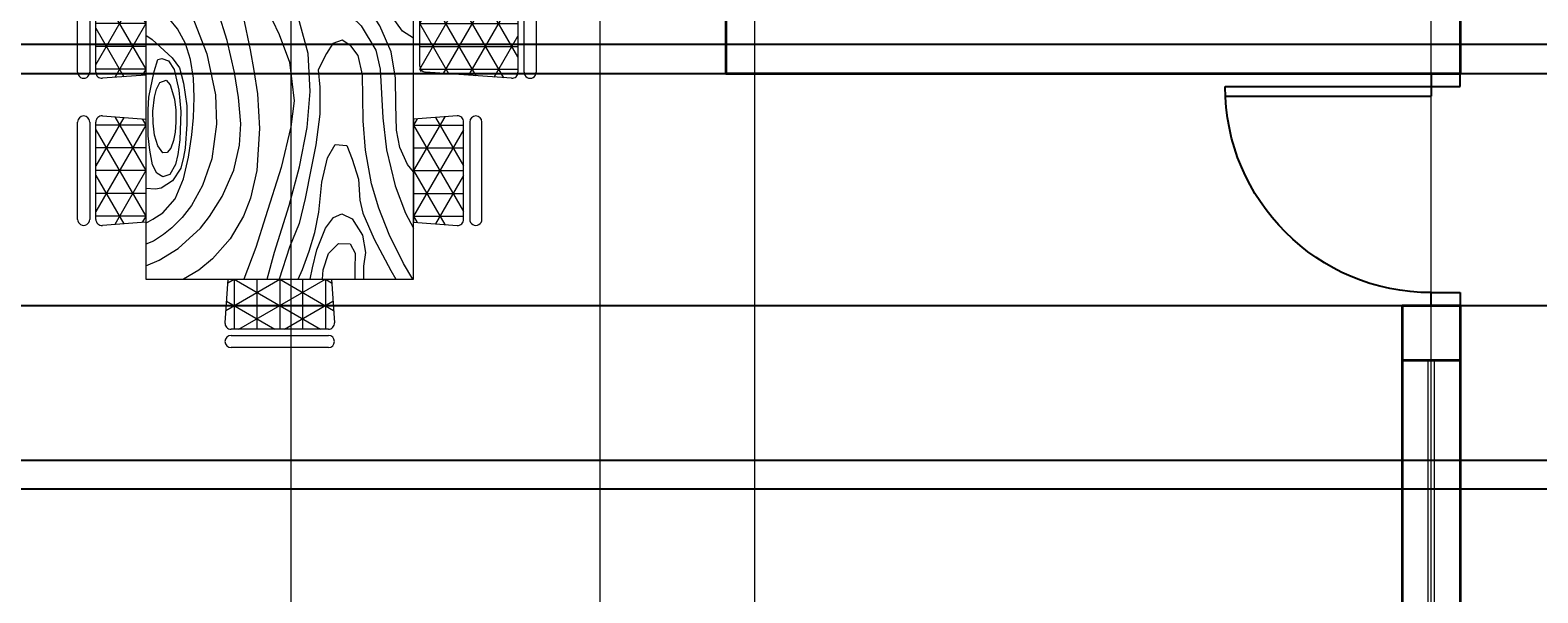
# Model space of a CAD drawing. Units: inches. Extents: x 5716 to 6907, y 12769 to 13594.
# Tile 14 of 17: x 6414 to 6648, y 13105 to 13192. Entities that reach past the tile are written whole.
import ezdxf

# ---------------------------------------------------------------- set-up
doc = ezdxf.new("R2010")
doc.units = ezdxf.units.IN
for name, color, linetype, lineweight in [('A-ANNO-DIMS', 2, 'Continuous', 18), ('A-DOOR', 4, 'Continuous', 25), ('A-FURN', 8, 'Continuous', 18), ('A-GLAZ', 4, 'Continuous', 18), ('A-GRID', 8, 'Continuous', 13), ('A-WALL', 7, 'Continuous', 35)]:
    doc.layers.add(name, color=color, linetype=linetype, lineweight=lineweight)
doc.styles.get("Standard").update_dxf_attribs({"font": 'arial.ttf'})
doc.dimstyles.get("Standard").update_dxf_attribs({"dimtxt": 0.18, "dimasz": 0.18, "dimexe": 0.18, "dimexo": 0.0625, "dimgap": 0.09, "dimtad": 0, "dimtih": 1, "dimtoh": 1, "dimdec": 4, "dimzin": 0, "dimdsep": 46, "dimtxsty": 'Standard', "dimcen": 0.09, "dimadec": 0, "dimazin": 0, "dimtfac": 1, "dimtdec": 4, "dimtofl": 0, "dimtmove": 0, "dimatfit": 3, "dimfxl": 1, "dimtolj": 1, "dimtzin": 0, "dimarcsym": 0})

# ---------------------------------------------------------------- blocks, each defined once
blk = doc.blocks.new('A$C405465A0')
for p, q in [((1.1305, 2.1034), (1.5301, 2.1034)), ((1.5301, 2.0534), (1.1305, 2.0534)), ((1.1304, 1.6481), (1.1055, 2.0017)), ((1.279, 2.0284), (1.1105, 1.9312)), ((1.4665, 2.0284), (1.1178, 1.8271)), ((1.1305, 2.0284), (1.5301, 2.0284)), ((1.1428, 1.625), (1.1428, 2.0284)), ((1.5427, 1.8271), (1.1941, 2.0284)), ((1.2365, 1.625), (1.2365, 2.0284)), ((1.3303, 1.625), (1.3303, 2.0284)), ((1.5501, 1.9312), (1.3816, 2.0284)), ((1.424, 1.625), (1.424, 2.0284)), ((1.5178, 1.625), (1.5178, 2.0284)), ((1.555, 2.0017), (1.5301, 1.6481)), ((1.5354, 1.7231), (1.1078, 1.97)), ((1.5528, 1.97), (1.1252, 1.7231)), ((0.9452, 1.8803), (0.5455, 1.8803)), ((2.1342, 1.8803), (1.7345, 1.8803)), ((0.5268, 1.6904), (0.7259, 1.8053)), ((0.5455, 1.8303), (0.9452, 1.8303)), ((0.9452, 1.8053), (0.5455, 1.8053)), ((0.5578, 1.6), (0.5578, 1.8053)), ((0.5578, 1.6), (0.9134, 1.8053)), ((0.5773, 1.8053), (0.9328, 1.6)), ((0.6516, 1.6), (0.6516, 1.8053)), ((0.7453, 1.6), (0.7453, 1.8053)), ((0.7648, 1.8053), (0.9639, 1.6904)), ((0.8391, 1.6), (0.8391, 1.8053)), ((0.9328, 1.6), (0.9328, 1.8053)), ((1.5178, 1.625), (1.1157, 1.8572)), ((1.5449, 1.8572), (1.1428, 1.625)), ((1.7158, 1.6904), (1.9149, 1.8053)), ((1.7345, 1.8303), (2.1342, 1.8303)), ((2.1342, 1.8053), (1.7345, 1.8053)), ((1.7468, 1.6), (1.7468, 1.8053)), ((1.7468, 1.6), (2.1024, 1.8053)), ((1.7663, 1.8053), (2.1218, 1.6)), ((1.8406, 1.6), (1.8406, 1.8053)), ((1.9343, 1.6), (1.9343, 1.8053)), ((1.9538, 1.8053), (2.1529, 1.6904)), ((2.0281, 1.6), (2.0281, 1.8053)), ((2.1218, 1.6), (2.1218, 1.8053)), ((0.5206, 1.7786), (0.5332, 1.6)), ((0.9575, 1.6), (0.9701, 1.7786)), ((1.3303, 1.625), (1.1237, 1.7443)), ((1.5369, 1.7443), (1.3303, 1.625)), ((1.7096, 1.7786), (1.7222, 1.6)), ((2.1465, 1.6), (2.1591, 1.7786)), ((0.5242, 1.7277), (0.7453, 1.6)), ((0.7453, 1.6), (0.9665, 1.7277)), ((1.7132, 1.7277), (1.9343, 1.6)), ((1.9343, 1.6), (2.1555, 1.7277)), ((0.5321, 1.6149), (0.5578, 1.6)), ((0.9328, 1.6), (0.9586, 1.6149)), ((1.1428, 1.625), (1.1316, 1.6315)), ((1.5052, 1.625), (1.1554, 1.625)), ((1.529, 1.6315), (1.5178, 1.625)), ((1.7211, 1.6149), (1.7468, 1.6)), ((2.1218, 1.6), (2.1476, 1.6149)), ((2.3803, 1.6), (0.2803, 1.6)), ((0.2803, 1.6), (0.2803, 0.5)), ((0.3956, 1.553), (0.3856, 1.5163)), ((0.4356, 1.5842), (0.3956, 1.553)), ((0.5827, 1.5379), (0.4356, 1.5842)), ((0.5332, 1.6), (0.9575, 1.6)), ((0.7152, 1.6), (0.7236, 1.5766)), ((0.7236, 1.5766), (0.7578, 1.4998)), ((0.9055, 1.5469), (0.8836, 1.6)), ((1.0212, 1.6), (1.0194, 1.5656)), ((1.0194, 1.5656), (1.026, 1.5003)), ((1.1178, 1.5243), (1.1269, 1.5706)), ((1.1269, 1.5706), (1.1432, 1.6)), ((1.1887, 1.5196), (1.1922, 1.5507)), ((1.1922, 1.5507), (1.214, 1.6)), ((1.3616, 1.5541), (1.3027, 1.5125)), ((1.3907, 1.6), (1.3616, 1.5541)), ((1.7222, 1.6), (2.1465, 1.6)), ((1.9093, 1.5754), (1.8386, 1.5427)), ((1.9386, 1.6), (1.9093, 1.5754)), ((1.9962, 1.5248), (2.1086, 1.5664)), ((2.1086, 1.5664), (2.17, 1.6)), ((2.3153, 1.558), (2.1962, 1.4994)), ((2.3803, 1.5967), (2.3153, 1.558)), ((2.3803, 0.5), (2.3803, 1.6)), ((0.3856, 1.5163), (0.4538, 1.4363)), ((0.4482, 1.5094), (0.4582, 1.5336)), ((0.4595, 1.4847), (0.4482, 1.5094)), ((0.4582, 1.5336), (0.5016, 1.5339)), ((0.5016, 1.5339), (0.54, 1.5204)), ((0.54, 1.5204), (0.5786, 1.5)), ((0.5786, 1.5), (0.6151, 1.4744)), ((0.6365, 1.5019), (0.5827, 1.5379)), ((0.7193, 1.4377), (0.6365, 1.5019)), ((0.7578, 1.4998), (0.7752, 1.4525)), ((0.9296, 1.4669), (0.9055, 1.5469)), ((1.026, 1.5003), (1.0343, 1.4559)), ((1.1128, 1.4699), (1.1178, 1.5243)), ((1.2089, 1.4946), (1.1887, 1.5196)), ((1.2618, 1.4976), (1.2089, 1.4946)), ((1.3027, 1.5125), (1.2618, 1.4976)), ((1.446, 1.5079), (1.3392, 1.4609)), ((1.5543, 1.5261), (1.446, 1.5079)), ((1.6627, 1.5271), (1.5543, 1.5261)), ((1.7679, 1.5301), (1.6627, 1.5271)), ((1.717, 1.474), (1.8488, 1.4892)), ((1.8386, 1.5427), (1.7679, 1.5301)), ((1.8488, 1.4892), (1.9962, 1.5248)), ((2.1962, 1.4994), (2.0887, 1.4564)), ((2.215, 1.4381), (2.3447, 1.5068)), ((2.3447, 1.5068), (2.3803, 1.5269)), ((0.3744, 1.3943), (0.2803, 1.458)), ((0.4538, 1.4363), (0.5034, 1.394)), ((0.4876, 1.4521), (0.4595, 1.4847)), ((0.5099, 1.4328), (0.4876, 1.4521)), ((0.5366, 1.4137), (0.5099, 1.4328)), ((0.6151, 1.4744), (0.6557, 1.4351)), ((0.6557, 1.4351), (0.6746, 1.4025)), ((0.7442, 1.4091), (0.7193, 1.4377)), ((0.7752, 1.4525), (0.7871, 1.4053)), ((0.9436, 1.385), (0.9296, 1.4669)), ((1.0343, 1.4559), (1.0488, 1.3883)), ((1.1133, 1.4295), (1.1128, 1.4699)), ((1.1222, 1.3821), (1.1133, 1.4295)), ((1.3392, 1.4609), (1.2655, 1.4131)), ((1.3398, 1.3841), (1.4396, 1.445)), ((1.4396, 1.445), (1.5179, 1.4625)), ((1.5179, 1.4625), (1.717, 1.474)), ((1.9879, 1.4268), (1.8502, 1.4019)), ((2.0887, 1.4564), (1.9879, 1.4268)), ((2.1089, 1.3912), (2.215, 1.4381)), ((0.4543, 1.3479), (0.3744, 1.3943)), ((0.5034, 1.394), (0.551, 1.3648)), ((0.5694, 1.3947), (0.5366, 1.4137)), ((0.551, 1.3648), (0.5952, 1.3458)), ((0.597, 1.3823), (0.5694, 1.3947)), ((0.6281, 1.3731), (0.597, 1.3823)), ((0.654, 1.3714), (0.6281, 1.3731)), ((0.674, 1.3825), (0.654, 1.3714)), ((0.6746, 1.4025), (0.674, 1.3825)), ((0.746, 1.3555), (0.7442, 1.4091)), ((0.7898, 1.3706), (0.7722, 1.3216)), ((0.7871, 1.4053), (0.7898, 1.3706)), ((0.9447, 1.3133), (0.9436, 1.385)), ((1.0488, 1.3883), (1.0626, 1.2943)), ((1.1508, 1.3537), (1.1222, 1.3821)), ((1.2034, 1.3712), (1.1508, 1.3537)), ((1.2655, 1.4131), (1.2034, 1.3712)), ((1.2659, 1.3078), (1.3398, 1.3841)), ((1.4616, 1.3726), (1.4211, 1.3426)), ((1.5407, 1.3902), (1.4616, 1.3726)), ((1.6315, 1.3907), (1.5407, 1.3902)), ((1.7291, 1.3922), (1.6315, 1.3907)), ((1.8502, 1.4019), (1.7291, 1.3922)), ((1.8869, 1.3472), (1.9689, 1.3731)), ((1.9689, 1.3731), (2.0551, 1.3789)), ((2.0551, 1.3789), (2.1089, 1.3912)), ((2.1327, 1.3477), (2.1998, 1.3905)), ((2.1998, 1.3905), (2.271, 1.4021)), ((2.271, 1.4021), (2.3264, 1.3943)), ((2.3264, 1.3943), (2.3803, 1.3943)), ((0.2803, 1.3424), (0.3226, 1.3046)), ((0.3226, 1.3046), (0.3891, 1.2586)), ((0.523, 1.3203), (0.4543, 1.3479)), ((0.6007, 1.301), (0.523, 1.3203)), ((0.5952, 1.3458), (0.6524, 1.335)), ((0.6623, 1.3018), (0.6007, 1.301)), ((0.6524, 1.335), (0.7159, 1.3352)), ((0.7385, 1.3018), (0.6623, 1.3018)), ((0.7159, 1.3352), (0.746, 1.3555)), ((0.7722, 1.3216), (0.7385, 1.3018)), ((0.9305, 1.2479), (0.9447, 1.3133)), ((1.1689, 1.1968), (1.2659, 1.3078)), ((1.4211, 1.3426), (1.398, 1.3071)), ((1.398, 1.3071), (1.412, 1.2681)), ((1.8267, 1.2783), (1.8309, 1.3257)), ((1.8309, 1.3257), (1.8869, 1.3472)), ((2.1112, 1.3052), (2.1327, 1.3477)), ((2.1264, 1.2714), (2.1112, 1.3052)), ((2.2336, 1.2914), (2.2346, 1.3391)), ((2.2346, 1.3391), (2.2726, 1.3593)), ((2.2726, 1.3593), (2.339, 1.3581)), ((2.339, 1.3581), (2.3803, 1.3581)), ((0, 1.2499), (0, 0.8502)), ((0.05, 0.8502), (0.05, 1.2499)), ((0.075, 1.0695), (0.19, 1.2686)), ((0.075, 1.2499), (0.075, 0.8502)), ((0.2803, 1.2622), (0.1018, 1.2748)), ((0.2803, 1.05), (0.1526, 1.2712)), ((0.2803, 1.2375), (0.2654, 1.2633)), ((0.3797, 1.2052), (0.2803, 1.2816)), ((0.2803, 0.8379), (0.2803, 1.2622)), ((0.2803, 1.2498), (0.478, 1.1251)), ((0.3891, 1.2586), (0.4808, 1.2074)), ((0.8894, 1.1911), (0.9305, 1.2479)), ((1.06, 1.2384), (1.0402, 1.1815)), ((1.0626, 1.2943), (1.06, 1.2384)), ((1.412, 1.2681), (1.4535, 1.2416)), ((1.4535, 1.2416), (1.5203, 1.2085)), ((1.8814, 1.2462), (1.8267, 1.2783)), ((1.9819, 1.2225), (1.8814, 1.2462)), ((2.171, 1.2386), (2.1264, 1.2714)), ((2.2593, 1.2028), (2.171, 1.2386)), ((2.2746, 1.2504), (2.2336, 1.2914)), ((2.3417, 1.2285), (2.2746, 1.2504)), ((2.3803, 1.2622), (2.5588, 1.2748)), ((2.3803, 1.05), (2.508, 1.2712)), ((2.3803, 1.2375), (2.3951, 1.2633)), ((2.3803, 0.8379), (2.3803, 1.2622)), ((2.5856, 1.0695), (2.4706, 1.2686)), ((2.5856, 1.2499), (2.5856, 0.8502)), ((2.6106, 0.8502), (2.6106, 1.2499)), ((2.6606, 1.2499), (2.6606, 0.8502)), ((0.2803, 1.2375), (0.075, 1.2375)), ((0.075, 0.882), (0.2803, 1.2375)), ((0.2803, 0.8625), (0.075, 1.2181)), ((0.3728, 1.1548), (0.2803, 1.2123)), ((0.4682, 1.1454), (0.3797, 1.2052)), ((0.4808, 1.2074), (0.5771, 1.1712)), ((0.8213, 1.159), (0.8894, 1.1911)), ((1.0402, 1.1815), (0.9932, 1.1252)), ((1.0809, 1.1136), (1.1689, 1.1968)), ((1.5203, 1.2085), (1.5912, 1.2143)), ((1.5912, 1.2143), (1.7027, 1.2151)), ((1.7027, 1.2151), (1.8282, 1.1987)), ((1.8282, 1.1987), (1.9236, 1.1792)), ((1.9236, 1.1792), (2.049, 1.1552)), ((2.1048, 1.2108), (1.9819, 1.2225)), ((2.1888, 1.194), (2.1048, 1.2108)), ((2.2653, 1.1704), (2.1888, 1.194)), ((2.3339, 1.1841), (2.2593, 1.2028)), ((2.3803, 1.1754), (2.3339, 1.1841)), ((2.3803, 1.226), (2.3417, 1.2285)), ((2.3803, 1.2375), (2.5856, 1.2375)), ((2.5856, 0.882), (2.3803, 1.2375)), ((2.3803, 0.8625), (2.5856, 1.2181)), ((0.2803, 1.1438), (0.075, 1.1438)), ((0.2803, 1.1471), (0.3609, 1.0879)), ((0.4405, 1.1078), (0.3728, 1.1548)), ((0.5225, 1.114), (0.4682, 1.1454)), ((0.478, 1.1251), (0.576, 1.067)), ((0.5771, 1.1712), (0.7161, 1.1491)), ((0.7161, 1.1491), (0.8213, 1.159)), ((0.9932, 1.1252), (0.9121, 1.0739)), ((1.3237, 1.1316), (1.2549, 1.1012)), ((1.4537, 1.1662), (1.3237, 1.1316)), ((1.6097, 1.1755), (1.4537, 1.1662)), ((1.757, 1.1624), (1.6097, 1.1755)), ((1.9184, 1.131), (1.757, 1.1624)), ((2.0769, 1.0887), (1.9184, 1.131)), ((2.049, 1.1552), (2.1515, 1.1303)), ((2.1515, 1.1303), (2.2486, 1.0908)), ((2.3396, 1.1432), (2.2653, 1.1704)), ((2.3803, 1.126), (2.3396, 1.1432)), ((2.3803, 1.1438), (2.5856, 1.1438)), ((0.3609, 1.0879), (0.5015, 1.0099)), ((0.5402, 1.0464), (0.4405, 1.1078)), ((0.5954, 1.0801), (0.5225, 1.114)), ((0.576, 1.067), (0.7146, 1.0163)), ((0.6603, 1.0585), (0.5954, 1.0801)), ((0.7308, 1.0454), (0.6603, 1.0585)), ((0.863, 1.056), (0.7897, 1.0439)), ((0.9121, 1.0739), (0.863, 1.056)), ((0.9069, 1.0237), (0.9908, 1.0561)), ((0.9908, 1.0561), (1.0809, 1.1136)), ((1.2549, 1.1012), (1.1432, 1.0368)), ((1.3755, 1.0479), (1.4887, 1.0901)), ((1.4887, 1.0901), (1.6473, 1.1088)), ((1.6473, 1.1088), (1.7544, 1.0961)), ((1.7544, 1.0961), (1.9207, 1.0564)), ((1.9207, 1.0564), (2.1244, 0.9922)), ((2.2686, 1.0282), (2.0769, 1.0887)), ((2.2486, 1.0908), (2.3803, 1.048)), ((0.2803, 1.05), (0.075, 1.05)), ((0.19, 0.8315), (0.075, 1.0306)), ((0.1526, 0.8289), (0.2803, 1.05)), ((0.3078, 1.029), (0.2803, 1.0458)), ((0.346, 1.0052), (0.3078, 1.029)), ((0.4051, 0.9771), (0.346, 1.0052)), ((0.5015, 1.0099), (0.6086, 0.961)), ((0.6261, 1.0028), (0.5402, 1.0464)), ((0.7415, 0.9604), (0.6261, 1.0028)), ((0.7146, 1.0163), (0.7979, 1.0084)), ((0.7897, 1.0439), (0.7308, 1.0454)), ((0.7979, 1.0084), (0.9069, 1.0237)), ((1.1432, 1.0368), (1.0559, 0.9876)), ((1.1244, 0.9348), (1.2543, 0.9907)), ((1.2543, 0.9907), (1.3755, 1.0479)), ((2.1244, 0.9922), (2.2495, 0.9522)), ((2.3803, 0.9983), (2.2686, 1.0282)), ((2.3803, 1.05), (2.5856, 1.05)), ((2.508, 0.8289), (2.3803, 1.05)), ((2.4706, 0.8315), (2.5856, 1.0306)), ((0.2803, 0.9563), (0.075, 0.9563)), ((0.4579, 0.9575), (0.4051, 0.9771)), ((0.5195, 0.9378), (0.4579, 0.9575)), ((0.5818, 0.918), (0.5195, 0.9378)), ((0.6086, 0.961), (0.7339, 0.9201)), ((0.8579, 0.9417), (0.7415, 0.9604)), ((0.958, 0.9508), (0.8579, 0.9417)), ((1.0559, 0.9876), (0.958, 0.9508)), ((0.9714, 0.9002), (1.1244, 0.9348)), ((1.4378, 0.9282), (1.5224, 0.9439)), ((1.5224, 0.9439), (1.6187, 0.9581)), ((1.6187, 0.9581), (1.7607, 0.9676)), ((1.7607, 0.9676), (1.9339, 0.9563)), ((1.9339, 0.9563), (2.0478, 0.9301)), ((2.0478, 0.9301), (2.1209, 0.9013)), ((2.2495, 0.9522), (2.3803, 0.9025)), ((2.3803, 0.9563), (2.5856, 0.9563)), ((0.309, 0.9074), (0.2803, 0.9224)), ((0.342, 0.8943), (0.309, 0.9074)), ((0.3823, 0.8837), (0.342, 0.8943)), ((0.4349, 0.876), (0.3823, 0.8837)), ((0.4843, 0.8652), (0.4349, 0.876)), ((0.6352, 0.8954), (0.5818, 0.918)), ((0.6712, 0.8671), (0.6352, 0.8954)), ((0.6805, 0.8424), (0.6712, 0.8671)), ((0.7339, 0.9201), (0.8463, 0.9008)), ((0.8463, 0.9008), (0.9714, 0.9002)), ((1.1125, 0.8545), (1.224, 0.8829)), ((1.224, 0.8829), (1.301, 0.9003)), ((1.301, 0.9003), (1.4378, 0.9282)), ((1.6341, 0.8806), (1.5313, 0.864)), ((1.7415, 0.8904), (1.6341, 0.8806)), ((1.8296, 0.8853), (1.7415, 0.8904)), ((1.9317, 0.8609), (1.8296, 0.8853)), ((2.1209, 0.9013), (2.214, 0.8459)), ((0.2803, 0.8625), (0.075, 0.8625)), ((0.1018, 0.8253), (0.2803, 0.8379)), ((0.2654, 0.8368), (0.2803, 0.8625)), ((0.5229, 0.85), (0.4843, 0.8652)), ((0.5441, 0.8372), (0.5229, 0.85)), ((0.5622, 0.8164), (0.5441, 0.8372)), ((0.5634, 0.7968), (0.5622, 0.8164)), ((0.6434, 0.7666), (0.675, 0.8159)), ((0.675, 0.8159), (0.6805, 0.8424)), ((0.9468, 0.8025), (1.1125, 0.8545)), ((1.3995, 0.834), (1.2818, 0.7979)), ((1.5313, 0.864), (1.3995, 0.834)), ((2.0406, 0.8138), (1.9317, 0.8609)), ((2.1229, 0.7618), (2.0406, 0.8138)), ((2.214, 0.8459), (2.297, 0.7736)), ((2.3803, 0.8625), (2.5856, 0.8625)), ((2.3951, 0.8368), (2.3803, 0.8625)), ((2.5588, 0.8253), (2.3803, 0.8379)), ((0.4801, 0.7185), (0.5313, 0.7537)), ((0.5313, 0.7537), (0.5562, 0.7809)), ((0.5562, 0.7809), (0.5634, 0.7968)), ((0.603, 0.7231), (0.6434, 0.7666)), ((0.6995, 0.6921), (0.8288, 0.7556)), ((0.8288, 0.7556), (0.9468, 0.8025)), ((1.2818, 0.7979), (1.131, 0.7357)), ((1.2995, 0.6899), (1.4547, 0.7504)), ((1.4547, 0.7504), (1.6229, 0.7863)), ((1.6229, 0.7863), (1.7436, 0.7907)), ((1.7436, 0.7907), (1.8858, 0.7711)), ((1.8858, 0.7711), (1.9957, 0.7333)), ((2.1698, 0.724), (2.1229, 0.7618)), ((2.297, 0.7736), (2.3432, 0.7176)), ((0.3723, 0.6742), (0.4317, 0.6944)), ((0.4317, 0.6944), (0.4801, 0.7185)), ((0.499, 0.6426), (0.5568, 0.6828)), ((0.5568, 0.6828), (0.603, 0.7231)), ((0.6181, 0.6464), (0.6995, 0.6921)), ((1.131, 0.7357), (0.9946, 0.6604)), ((1.2062, 0.6433), (1.2995, 0.6899)), ((1.4772, 0.6838), (1.4124, 0.6631)), ((1.554, 0.696), (1.4772, 0.6838)), ((1.6333, 0.6993), (1.554, 0.696)), ((1.7153, 0.696), (1.6333, 0.6993)), ((1.7865, 0.6892), (1.7153, 0.696)), ((1.8794, 0.6748), (1.7865, 0.6892)), ((1.9957, 0.7333), (2.0772, 0.6873)), ((2.0772, 0.6873), (2.1261, 0.6491)), ((2.2541, 0.6328), (2.1698, 0.724)), ((2.3432, 0.7176), (2.3803, 0.6555)), ((0.2803, 0.6573), (0.312, 0.6622)), ((0.312, 0.6622), (0.3723, 0.6742)), ((0.4497, 0.615), (0.499, 0.6426)), ((0.5546, 0.6082), (0.6181, 0.6464)), ((0.9946, 0.6604), (0.8746, 0.5766)), ((1.1078, 0.5882), (1.2062, 0.6433)), ((1.3518, 0.6302), (1.3133, 0.5983)), ((1.4124, 0.6631), (1.3518, 0.6302)), ((1.4712, 0.6079), (1.5115, 0.6388)), ((1.5115, 0.6388), (1.5744, 0.6543)), ((1.5188, 0.6159), (1.6031, 0.6361)), ((1.5744, 0.6543), (1.6677, 0.668)), ((1.6031, 0.6361), (1.6918, 0.6436)), ((1.641, 0.6183), (1.6861, 0.6235)), ((1.6677, 0.668), (1.7434, 0.6684)), ((1.6861, 0.6235), (1.7353, 0.624)), ((1.6918, 0.6436), (1.8075, 0.6404)), ((1.7353, 0.624), (1.7765, 0.6204)), ((1.7434, 0.6684), (1.8417, 0.6617)), ((1.7765, 0.6204), (1.811, 0.6136)), ((1.8075, 0.6404), (1.8682, 0.6312)), ((1.8417, 0.6617), (1.8785, 0.6547)), ((1.8682, 0.6312), (1.909, 0.622)), ((1.8785, 0.6547), (1.9243, 0.6434)), ((1.9674, 0.6548), (1.8794, 0.6748)), ((1.909, 0.622), (1.9497, 0.5991)), ((1.9243, 0.6434), (1.9761, 0.6102)), ((2.0494, 0.621), (1.9674, 0.6548)), ((2.1071, 0.5697), (2.0494, 0.621)), ((2.1261, 0.6491), (2.1688, 0.6067)), ((2.3022, 0.5551), (2.2541, 0.6328)), ((0.2803, 0.5477), (0.3159, 0.5583)), ((0.3159, 0.5583), (0.3813, 0.5837)), ((0.3813, 0.5837), (0.4497, 0.615)), ((0.4385, 0.5349), (0.5546, 0.6082)), ((0.8746, 0.5766), (0.8225, 0.5348)), ((1.0064, 0.5273), (1.1078, 0.5882)), ((1.2908, 0.5736), (1.2556, 0.52)), ((1.3133, 0.5983), (1.2908, 0.5736)), ((1.3959, 0.5264), (1.4712, 0.6079)), ((1.4736, 0.5658), (1.4828, 0.5927)), ((1.4775, 0.5489), (1.4736, 0.5658)), ((1.4828, 0.5927), (1.5188, 0.6159)), ((1.5621, 0.583), (1.5815, 0.6002)), ((1.572, 0.557), (1.5621, 0.583)), ((1.5815, 0.6002), (1.641, 0.6183)), ((1.811, 0.6136), (1.8414, 0.6025)), ((1.8611, 0.5702), (1.8321, 0.5488)), ((1.8414, 0.6025), (1.8603, 0.5873)), ((1.8603, 0.5873), (1.8611, 0.5702)), ((1.9595, 0.5705), (1.9448, 0.5456)), ((1.9497, 0.5991), (1.9595, 0.5705)), ((1.9761, 0.6102), (2.006, 0.5625)), ((2.006, 0.5625), (2.0103, 0.5395)), ((2.1338, 0.529), (2.1071, 0.5697)), ((2.1688, 0.6067), (2.197, 0.5721)), ((2.197, 0.5721), (2.2242, 0.5314)), ((0.2803, 0.5), (2.3803, 0.5)), ((0.3857, 0.5), (0.4385, 0.5349)), ((0.8225, 0.5348), (0.7878, 0.5)), ((0.9657, 0.5), (1.0064, 0.5273)), ((1.1055, 0.3215), (1.1181, 0.5)), ((1.1091, 0.3724), (1.3303, 0.5)), ((1.1171, 0.4852), (1.1428, 0.5)), ((1.1181, 0.5), (1.5425, 0.5)), ((1.1428, 0.5), (1.1428, 0.2948)), ((1.1428, 0.5), (1.4984, 0.2948)), ((1.1622, 0.2948), (1.5178, 0.5)), ((1.2365, 0.5), (1.2365, 0.2948)), ((1.2556, 0.52), (1.2455, 0.5)), ((1.3303, 0.5), (1.3303, 0.2948)), ((1.3303, 0.5), (1.5515, 0.3724)), ((1.3784, 0.5), (1.3959, 0.5264)), ((1.424, 0.5), (1.424, 0.2948)), ((1.5273, 0.534), (1.4775, 0.5489)), ((1.5178, 0.5), (1.5178, 0.2948)), ((1.5178, 0.5), (1.5435, 0.4852)), ((1.6327, 0.513), (1.5273, 0.534)), ((1.5425, 0.5), (1.555, 0.3215)), ((1.5997, 0.5436), (1.572, 0.557)), ((1.6329, 0.5353), (1.5997, 0.5436)), ((1.685, 0.5094), (1.6327, 0.513)), ((1.6895, 0.5294), (1.6329, 0.5353)), ((1.7331, 0.5091), (1.685, 0.5094)), ((1.7388, 0.53), (1.6895, 0.5294)), ((1.7096, 0.3215), (1.7222, 0.5)), ((1.7132, 0.3724), (1.9343, 0.5)), ((1.7211, 0.4852), (1.7468, 0.5)), ((1.7222, 0.5), (2.1465, 0.5)), ((1.7906, 0.5103), (1.7331, 0.5091)), ((1.7888, 0.5363), (1.7388, 0.53)), ((1.7468, 0.5), (1.7468, 0.2948)), ((1.7468, 0.5), (2.1024, 0.2948)), ((1.7663, 0.2948), (2.1218, 0.5)), ((1.8321, 0.5488), (1.7888, 0.5363)), ((1.8503, 0.5169), (1.7906, 0.5103)), ((1.8406, 0.5), (1.8406, 0.2948)), ((1.9108, 0.5271), (1.8503, 0.5169)), ((1.9448, 0.5456), (1.9108, 0.5271)), ((1.9343, 0.5), (1.9343, 0.2948)), ((1.9343, 0.5), (2.1555, 0.3724)), ((2.0103, 0.5395), (2.0069, 0.5)), ((2.0281, 0.5), (2.0281, 0.2948)), ((2.1218, 0.5), (2.1218, 0.2948)), ((2.1218, 0.5), (2.1476, 0.4852)), ((2.1506, 0.5), (2.1338, 0.529)), ((2.1465, 0.5), (2.1591, 0.3215)), ((2.2242, 0.5314), (2.2363, 0.5)), ((2.3248, 0.5), (2.3022, 0.5551)), ((0.5024, 0.1018), (0.5273, 0.4553)), ((0.5126, 0.2463), (0.9147, 0.4784)), ((0.5205, 0.3591), (0.7272, 0.4784)), ((0.5285, 0.4719), (0.5397, 0.4784)), ((0.5397, 0.4784), (0.5397, 0.075)), ((0.5397, 0.4784), (0.9417, 0.2463)), ((0.5522, 0.4784), (0.9021, 0.4784)), ((0.6334, 0.4784), (0.6334, 0.075)), ((0.7272, 0.4784), (0.7272, 0.075)), ((0.7272, 0.4784), (0.9338, 0.3591)), ((0.8209, 0.4784), (0.8209, 0.075)), ((0.9147, 0.4784), (0.9147, 0.075)), ((0.9147, 0.4784), (0.9258, 0.4719)), ((0.927, 0.4553), (0.9519, 0.1018)), ((0.5046, 0.1334), (0.9323, 0.3803)), ((0.522, 0.3803), (0.9497, 0.1334)), ((1.1118, 0.4097), (1.3109, 0.2948)), ((1.3497, 0.2948), (1.5488, 0.4097)), ((1.7158, 0.4097), (1.9149, 0.2948)), ((1.9538, 0.2948), (2.1529, 0.4097)), ((0.5147, 0.2763), (0.8634, 0.075)), ((0.591, 0.075), (0.9396, 0.2763)), ((1.5301, 0.2948), (1.1305, 0.2948)), ((1.1305, 0.2698), (1.5301, 0.2698)), ((2.1342, 0.2948), (1.7345, 0.2948)), ((1.7345, 0.2698), (2.1342, 0.2698)), ((1.5301, 0.2198), (1.1305, 0.2198)), ((2.1342, 0.2198), (1.7345, 0.2198)), ((0.5074, 0.1723), (0.6759, 0.075)), ((0.7785, 0.075), (0.9469, 0.1723)), ((0.927, 0.075), (0.5273, 0.075)), ((0.5273, 0.05), (0.927, 0.05)), ((0.927, 0), (0.5273, 0))]:
    blk.add_line(p, q)
for centre, start, end in [((1.1305, 2.0784), 90, 270), ((1.5301, 2.0784), 270, 90), ((1.1305, 2.0034), 90, 184.02744), ((1.5301, 2.0034), 355.97256, 90), ((0.5455, 1.8553), 90, 270), ((0.9452, 1.8553), 270, 90), ((1.7345, 1.8553), 90, 270), ((2.1342, 1.8553), 270, 90), ((0.5455, 1.7803), 90, 184.02744), ((0.9452, 1.7803), 355.97256, 90), ((1.7345, 1.7803), 90, 184.02744), ((2.1342, 1.7803), 355.97256, 90), ((1.1554, 1.65), 184.39871, 270), ((1.5052, 1.65), 270, 355.60129), ((0.025, 1.2499), 0, 180), ((0.1, 1.2499), 85.97256, 180), ((2.5606, 1.2499), 0, 94.02744), ((2.6356, 1.2499), 0, 180), ((0.025, 0.8502), 180, 0), ((0.1, 0.8502), 180, 274.02744), ((2.5606, 0.8502), 265.97256, 0), ((2.6356, 0.8502), 180, 0), ((0.5522, 0.4534), 90, 175.60129), ((0.9021, 0.4534), 4.39871, 90), ((1.1305, 0.3198), 175.97256, 270), ((1.5301, 0.3198), 270, 4.02744), ((1.7345, 0.3198), 175.97256, 270), ((2.1342, 0.3198), 270, 4.02744), ((1.1305, 0.2448), 90, 270), ((1.5301, 0.2448), 270, 90), ((1.7345, 0.2448), 90, 270), ((2.1342, 0.2448), 270, 90), ((0.5273, 0.1), 175.97256, 270), ((0.927, 0.1), 270, 4.02744), ((0.5273, 0.025), 90, 270), ((0.927, 0.025), 270, 90)]:
    blk.add_arc(centre, 0.025, start, end)
blk = doc.blocks.new('DOOR-SWING-36IN')
for p, q in [((0, 32), (0, 0)), ((1.5, 31.96), (1.5, 0)), ((-2, 0), (0, 0)), ((0, 0), (0, -4.5)), ((0, 0), (1.5, 0)), ((34, 0), (32, 0)), ((32, 0), (32, -4.5)), ((0, -4.5), (-2, -4.5)), ((32, -4.5), (34, -4.5))]:
    blk.add_line(p, q)
blk.add_arc((0, 0), 32, 0, 90)
blk = doc.blocks.new('WIN-GLAZING-48IN')
for p, q in [((0, 0), (0, 48)), ((1, 0), (1, 48))]:
    blk.add_line(p, q)
blk = doc.blocks.new('*D60')
at = {"layer": 'A-ANNO-DIMS', "color": 0, "lineweight": -2, "transparency": 16777216}
for p, q in [((6736.67, 13201.65), (5716.04, 13201.65)), ((5716.22, 13201.47), (5716.22, 13195.83)), ((5716.22, 13189.83), (5716.22, 13195.47)), ((6827.78, 13189.65), (5716.04, 13189.65))]:
    blk.add_line(p, q, dxfattribs=at)
at = {"layer": 'A-ANNO-DIMS', "color": 0, "transparency": 16777216}
for points in [[(5716.19, 13201.47), (5716.25, 13201.47), (5716.22, 13201.65)], [(5716.19, 13189.83), (5716.25, 13189.83), (5716.22, 13189.65)]]:
    blk.add_solid(points, dxfattribs=at)
at = {"layer": 'Defpoints', "color": 0, "transparency": 16777216}
for p in [(6736.73, 13201.65), (5716.22, 13189.65), (6827.84, 13189.65)]:
    blk.add_point(p, dxfattribs=at)
at = {"layer": 'A-ANNO-DIMS', "color": 0, "transparency": 16777216, "insert": (5716.22, 13195.65), "char_height": 0.18, "attachment_point": 5}
blk.add_mtext('\\A1;12', dxfattribs=at)
blk = doc.blocks.new('*D61')
at = {"layer": 'A-ANNO-DIMS', "color": 0, "lineweight": -2, "transparency": 16777216}
for p, q in [((6827.78, 13189.65), (5716.04, 13189.65)), ((5716.22, 13189.47), (5716.22, 13155.33)), ((5716.22, 13120.83), (5716.22, 13154.97)), ((6736.67, 13120.65), (5716.04, 13120.65))]:
    blk.add_line(p, q, dxfattribs=at)
at = {"layer": 'A-ANNO-DIMS', "color": 0, "transparency": 16777216}
for points in [[(5716.19, 13189.47), (5716.25, 13189.47), (5716.22, 13189.65)], [(5716.19, 13120.83), (5716.25, 13120.83), (5716.22, 13120.65)]]:
    blk.add_solid(points, dxfattribs=at)
at = {"layer": 'Defpoints', "color": 0, "transparency": 16777216}
for p in [(6827.84, 13189.65), (5716.22, 13120.65), (6736.73, 13120.65)]:
    blk.add_point(p, dxfattribs=at)
at = {"layer": 'A-ANNO-DIMS', "color": 0, "transparency": 16777216, "insert": (5716.22, 13155.15), "char_height": 0.18, "attachment_point": 5}
blk.add_mtext('\\A1;69', dxfattribs=at)
blk = doc.blocks.new('*D62')
at = {"layer": 'A-ANNO-DIMS', "color": 0, "lineweight": -2, "transparency": 16777216}
for p, q in [((6736.67, 13120.65), (5716.04, 13120.65)), ((5716.22, 13120.47), (5716.22, 13100.33)), ((5716.22, 13079.83), (5716.22, 13099.97)), ((6736.67, 13079.65), (5716.04, 13079.65))]:
    blk.add_line(p, q, dxfattribs=at)
at = {"layer": 'A-ANNO-DIMS', "color": 0, "transparency": 16777216}
for points in [[(5716.19, 13120.47), (5716.25, 13120.47), (5716.22, 13120.65)], [(5716.19, 13079.83), (5716.25, 13079.83), (5716.22, 13079.65)]]:
    blk.add_solid(points, dxfattribs=at)
at = {"layer": 'Defpoints', "color": 0, "transparency": 16777216}
for p in [(6736.73, 13120.65), (5716.22, 13079.65), (6736.73, 13079.65)]:
    blk.add_point(p, dxfattribs=at)
at = {"layer": 'A-ANNO-DIMS', "color": 0, "transparency": 16777216, "insert": (5716.22, 13100.15), "char_height": 0.18, "attachment_point": 5}
blk.add_mtext('\\A1;41', dxfattribs=at)
blk = doc.blocks.new('*D69')
at = {"layer": 'A-ANNO-DIMS', "color": 0, "lineweight": -2, "transparency": 16777216}
for p, q in [((5828.09, 13149.15), (6907.26, 13149.15)), ((6907.08, 13148.97), (6907.08, 13137.33)), ((6907.08, 13125.33), (6907.08, 13136.97)), ((5828.09, 13125.15), (6907.26, 13125.15))]:
    blk.add_line(p, q, dxfattribs=at)
at = {"layer": 'A-ANNO-DIMS', "color": 0, "transparency": 16777216}
for points in [[(6907.05, 13148.97), (6907.11, 13148.97), (6907.08, 13149.15)], [(6907.05, 13125.33), (6907.11, 13125.33), (6907.08, 13125.15)]]:
    blk.add_solid(points, dxfattribs=at)
at = {"layer": 'Defpoints', "color": 0, "transparency": 16777216}
for p in [(5828.02, 13149.15), (6907.08, 13149.15), (5828.02, 13125.15)]:
    blk.add_point(p, dxfattribs=at)
at = {"layer": 'A-ANNO-DIMS', "color": 0, "transparency": 16777216, "insert": (6907.08, 13137.15), "char_height": 0.18, "attachment_point": 5}
blk.add_mtext('\\A1;24', dxfattribs=at)
blk = doc.blocks.new('*D74')
at = {"layer": 'A-ANNO-DIMS', "color": 0, "lineweight": -2, "transparency": 16777216}
for p, q in [((6188.09, 13185.15), (6907.26, 13185.15)), ((6907.08, 13184.97), (6907.08, 13167.33)), ((6907.08, 13149.33), (6907.08, 13166.97)), ((6188.09, 13149.15), (6907.26, 13149.15))]:
    blk.add_line(p, q, dxfattribs=at)
at = {"layer": 'A-ANNO-DIMS', "color": 0, "transparency": 16777216}
for points in [[(6907.05, 13184.97), (6907.11, 13184.97), (6907.08, 13185.15)], [(6907.05, 13149.33), (6907.11, 13149.33), (6907.08, 13149.15)]]:
    blk.add_solid(points, dxfattribs=at)
at = {"layer": 'Defpoints', "color": 0, "transparency": 16777216}
for p in [(6188.02, 13185.15), (6907.08, 13185.15), (6188.02, 13149.15)]:
    blk.add_point(p, dxfattribs=at)
at = {"layer": 'A-ANNO-DIMS', "color": 0, "transparency": 16777216, "insert": (6907.08, 13167.15), "char_height": 0.18, "attachment_point": 5}
blk.add_mtext('\\A1;36', dxfattribs=at)

msp = doc.modelspace()

# ---------------------------------------------------------------- linework, layer by layer
at = {"layer": 'A-GRID'}
for p, q in [((6454.91, 12841.15), (6454.91, 13514.96)), ((6502.91, 12841.15), (6502.91, 13514.96)), ((6526.91, 12841.15), (6526.91, 13514.96)), ((6631.91, 12841.15), (6631.91, 13514.96)), ((6267.41, 13189.65), (6827.84, 13189.65)), ((6267.41, 13120.65), (6736.73, 13120.65))]:
    msp.add_line(p, q, dxfattribs=at)
at = {"layer": 'A-WALL'}
for p, q in [((6636.41, 13440.15), (6636.41, 13185.15)), ((6522.41, 13290.15), (6522.41, 13185.15)), ((6522.41, 13185.15), (6636.41, 13185.15)), ((6627.41, 13149.15), (6627.41, 13084.15)), ((6627.41, 13149.15), (6636.41, 13149.15)), ((6636.41, 13149.15), (6636.41, 12934.15)), ((6627.41, 13140.65), (6636.41, 13140.65))]:
    msp.add_line(p, q, dxfattribs=at)

# ---------------------------------------------------------------- block references
at = {"layer": 'A-DOOR', "extrusion": (0, 0, -1), "zscale": -1, "rotation": 269.9999999999987}
msp.add_blockref('DOOR-SWING-36IN', (-6631.91, 13183.15), dxfattribs=at)
at = {"layer": 'A-FURN', "xscale": 37.79737452882042, "yscale": 37.79737452882042, "zscale": 37.79737452882042, "rotation": 270}
msp.add_blockref('A$C405465A0', (6413.46, 13243.2), dxfattribs=at)
at = {"layer": 'A-GLAZ'}
msp.add_blockref('WIN-GLAZING-48IN', (6631.41, 13092.65), dxfattribs=at)

# ---------------------------------------------------------------- dimensions: what is measured, and where the dimension line sits
at = {"layer": 'A-ANNO-DIMS'}
for base, p1, p2, picture, middle in [((5716.22, 13189.65), (6736.73, 13201.65), (6827.84, 13189.65), '*D60', (5716.22, 13195.65)), ((5716.22, 13120.65), (6827.84, 13189.65), (6736.73, 13120.65), '*D61', (5716.22, 13155.15)), ((6907.08, 13185.15), (6188.02, 13149.15), (6188.02, 13185.15), '*D74', (6907.08, 13167.15)), ((6907.08, 13149.15), (5828.02, 13125.15), (5828.02, 13149.15), '*D69', (6907.08, 13137.15)), ((5716.22, 13079.65), (6736.73, 13120.65), (6736.73, 13079.65), '*D62', (5716.22, 13100.15))]:
    dim = msp.add_linear_dim(base=base, p1=p1, p2=p2, angle=90, dimstyle='Standard', override={"dimdec": 0, "dimlfac": 1, "dimrnd": 0, "dimzin": 0, "dimdsep": 46, "dimlunit": 2}, dxfattribs=at)
    dim.commit()
    dim.dimension.update_dxf_attribs({"geometry": picture, "text_midpoint": middle})

doc.saveas('drawing.dxf')
